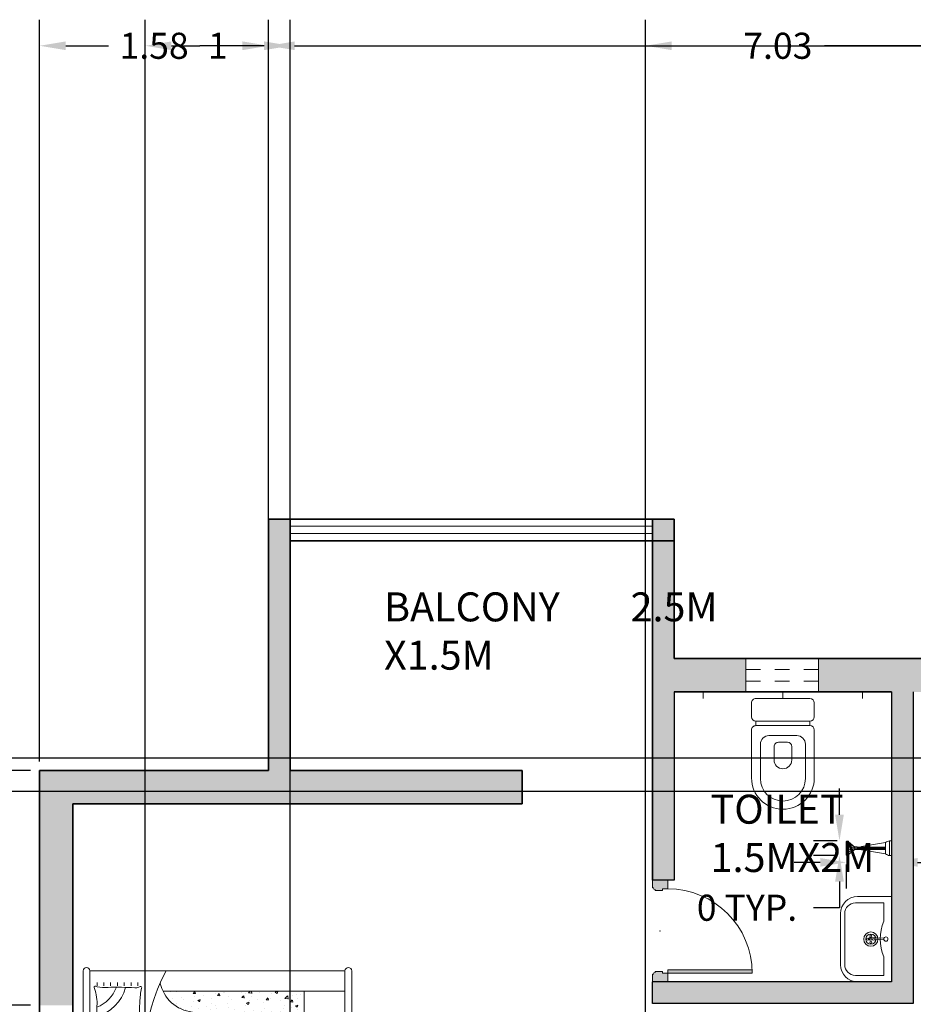
# Model space of a CAD drawing. Units: metres. Extents: x 2031 to 2061.8, y 1886.4 to 1909.8.
# Tile 6 of 10: x 2036.1 to 2042.3, y 1903 to 1909.8. Entities that reach past the tile are written whole.
import ezdxf

# ---------------------------------------------------------------- set-up
doc = ezdxf.new("R2010")
doc.units = ezdxf.units.M
doc.linetypes.add('DASHED', pattern=[0.75, 0.5, -0.25])
for name, color, linetype, lineweight in [('A-ANNO-DIMS', 2, 'Continuous', 18), ('A-AREA-IDEN', 7, 'Continuous', 18), ('A-FLOR-FIXT', 8, 'Continuous', 18), ('A-GLAZ-OVHD', 30, 'DASHED', 13), ('A-WALL-PATT', 252, 'Continuous', 13), ('doors & windows', 30, 'Continuous', 18), ('furniture', 24, 'Continuous', 13), ('grills', 5, 'Continuous', 13), ('inner walls', 4, 'Continuous', 25), ('windows', 30, 'Continuous', 18)]:
    doc.layers.add(name, color=color, linetype=linetype, lineweight=lineweight)
doc.layers.add('outer walls', color=1, linetype='Continuous', lineweight=35, plot=False)
doc.styles.get("Standard").update_dxf_attribs({"font": 'arial.ttf'})
doc.dimstyles.get("Standard").update_dxf_attribs({"dimtxt": 0.18, "dimasz": 0.18, "dimexe": 0.18, "dimexo": 0.0625, "dimgap": 0.09, "dimtad": 0, "dimtih": 1, "dimtoh": 1, "dimdec": 4, "dimzin": 0, "dimdsep": 46, "dimtxsty": 'Standard', "dimcen": 0.09, "dimadec": 0, "dimazin": 0, "dimtfac": 1, "dimtdec": 4, "dimtofl": 0, "dimtmove": 0, "dimatfit": 3, "dimfxl": 1, "dimtolj": 1, "dimtzin": 0, "dimarcsym": 0})

# ---------------------------------------------------------------- blocks, each defined once
blk = doc.blocks.new('D2')
at = {"layer": 'doors & windows'}
h = blk.add_hatch(dxfattribs=at)
h.set_pattern_fill('DOTS', color=256, scale=2, angle=180, style=0)
h.set_pattern_definition([(180, (0, -3.999999999998181), (-0.0625, -0.125), [0, -0.125])])
h.paths.add_polyline_path([(2.5, 1.819e-12), (3.5, 1.819e-12), (3.500000000001818, 24.97999199359535, 0.0100030022021123), (2.500000000001818, 25.00000000000182)])
h = blk.add_hatch(dxfattribs=at)
h.set_pattern_fill('DOTS', color=256, scale=2, angle=180, style=0)
h.set_pattern_definition([(180, (0, 0), (-0.0625, -0.125), [0, -0.125])])
edge = h.paths.add_edge_path()
edge.add_line((27.50000000000182, 1.819e-12), (27.50000000000182, -1.499999999998181))
edge.add_line((27.50000000000182, -1.499999999998181), (27.00000000000157, -1.499999999998181))
edge.add_line((27.00000000000157, -1.499999999998181), (27.00000000000039, -3.749999999998181))
edge.add_line((27.00000000000039, -3.749999999998181), (27.25, -3.749999999998181))
edge.add_arc((27.75893604593965, -3.741063954058532), 0.5090144907305875, 181.0059124648427, 268.9940875351573)
edge.add_line((27.75, -4.249999999998181), (27.75, -4.499999999998181))
edge.add_line((27.75, -4.499999999998181), (30.00000000000182, -4.499999999998181))
edge.add_line((30.00000000000182, -4.499999999998181), (30.00000000000182, 0))
edge.add_line((30.00000000000182, 0), (27.50000000000182, 1.819e-12))
edge = h.paths.add_edge_path()
edge.add_line((2.5, -1.499999999998181), (2.5, 1.819e-12))
edge.add_line((2.5, 1.819e-12), (1.819e-12, 0))
edge.add_line((1.819e-12, 0), (0, -4.499999999998181))
edge.add_line((0, -4.499999999998181), (2.250000000001548, -4.499999999998181))
edge.add_line((2.250000000001548, -4.499999999998181), (2.250000000001548, -4.249999999998181))
edge.add_arc((2.2410639540619, -3.741063954058532), 0.5090144907305875, 271.0059124648427, 358.9940875351573)
edge.add_line((2.750000000001548, -3.749999999998181), (3, -3.749999999998181))
edge.add_line((3, -3.749999999998181), (3, -1.499999999998181))
edge.add_line((3, -1.499999999998181), (2.5, -1.499999999998181))
for p, q in [((1.819e-12, 0), (0, -4.499999999998181)), ((30.00000000000182, 0), (30.00000000000182, -4.499999999998181))]:
    blk.add_line(p, q)
blk.add_lwpolyline([(3.5, 1.819e-12), (3.500000000001818, 25.00000000000182), (2.500000000001818, 25.00000000000182), (2.5, 1.819e-12)], close=True, dxfattribs=at)
for points in [[(3, -3.749999999998181), (3, -1.499999999998181), (2.5, -1.499999999998181), (2.5, 1.819e-12), (1.819e-12, 0)], [(27.00000000000039, -3.749999999998181), (27.00000000000182, -1.499999999998181), (27.50000000000182, -1.499999999998181), (27.50000000000182, 1.819e-12), (30, 0)], [(0, -4.499999999998181), (2.250000000001548, -4.499999999998181)], [(30, -4.499999999998181), (27.75, -4.499999999998181)]]:
    blk.add_lwpolyline(points, dxfattribs=at)
for points in [[(2.250000000001548, -4.499999999998181), (2.250000000001548, -4.249999999998181, 0.4039662087126686), (2.750000000001548, -3.749999999998181), (3.000000000001548, -3.749999999998181)], [(27.75, -4.499999999998181), (27.75, -4.249999999998181, -0.4039662087126686), (27.25, -3.749999999998181), (27, -3.749999999998181)]]:
    blk.add_lwpolyline(points, format="xyb", dxfattribs=at)
at = {"layer": 'doors & windows', "ltscale": 6}
blk.add_arc((2.5, 1.819e-12), 25, 0, 90, dxfattribs=at)
at = {"layer": 'doors & windows'}
blk.add_point((15, -2.24999999999909), dxfattribs=at)
blk = doc.blocks.new('wash basin 1')
for p, q in [((2.4e-15, 10), (-8, 10)), ((2.4e-15, 10), (-2.4e-15, -10)), ((-8.5, 8.5), (-1.851811242548834, 8.500000000000004)), ((-1.851811242548834, 8.500000000000004), (-1.851811242548897, 4.188089367671713)), ((-12, 6), (-12, -6.000000000000001)), ((-11, 6), (-11, -6.000000000000001)), ((-1.851811242548729, -8.5), (-1.851811242548728, -4.188089367671126)), ((-8.500000000000002, -8.500000000000002), (-1.851811242548729, -8.5)), ((-2.4e-15, -10), (-8.000000000000002, -10))]:
    blk.add_line(p, q)
blk.add_lwpolyline([(-1.829996854681013, 0.1082389988048371), (-5.253671435714977, 0.2462926470149123), (-5.229221238307189, -0.3815455523157976), (-1.804400006573047, -0.1898693366394459)])
for centre, radius in [((-4.868871099337752, 1.8e-15), 1.677439688297454), ((-4.868871099337752, 1.8e-15), 1.177439688297454), ((-5.631604960595723, 1.8e-15), 0.25), ((-4.873580145140294, 0.7523876361110525), 0.25), ((-4.868871099337752, 1.8e-15), 0.25), ((-4.194973017078154, 1.8e-15), 0.25), ((-1.341853106244229, 7.967e-13), 0.5), ((-4.868871099337752, -0.7188855560125376), 0.25)]:
    blk.add_circle(centre, radius)
for centre, radius, start, end in [((-8, 6), 4, 90, 180), ((-8.5, 6), 2.5, 90, 180), ((8.8933346853213, 5.103e-13), 11.53248687676786, 158.7058692194464, 201.2941307805559), ((-8.000000000000002, -6.000000000000001), 4, 180, 270), ((-8.500000000000002, -6.000000000000001), 2.5, 180, 270)]:
    blk.add_arc(centre, radius, start, end)
blk = doc.blocks.new('commode')
for p, q in [((-7.091161676878982, 19.40883832311374), (-7.091161676878982, 8.608954493363852)), ((-5.091161676878982, 11.8123055313481), (-5.091161676878982, 19.56719258349039)), ((5.091161676893534, 11.8123055313481), (5.091161676893534, 19.56719258349039)), ((7.091161676893534, 19.40883832311374), (7.091161676893534, 8.608954493363852)), ((-1.999999999985448, 12.37086546904174), (-1.999999999985448, 15.37086546904174)), ((2.000000000014551, 12.37086546904174), (2.000000000014551, 15.37086546904174)), ((-0.999999999985448, 11.37086546904174), (1.000000000014551, 11.37086546904174)), ((-3.149721614536247, 9.870865469041746), (3.149721614565351, 9.870865469041746)), ((-6.091161676878982, 7.608954493363853), (6.091161676893534, 7.608954493363853)), ((-6.091161676878982, 6.608954493363853), (-6.091161676878982, 7.608954493363851)), ((6.091161676893534, 7.608954493363854), (6.091161676893534, 6.608954493363853)), ((-7.091161676878982, 2.5), (-7.091161676878982, 5.608954493363853)), ((-6.091161676878982, 6.608954493363853), (6.091161676893534, 6.608954493363853)), ((7.091161676893534, 2.5), (7.091161676893534, 5.608954493363853)), ((-18, 1.5), (-18, 0)), ((-6.091161676878982, 1.5), (6.091161676893534, 1.5)), ((0, 1.5), (0, 0)), ((18, 1.5), (18, 0))]:
    blk.add_line(p, q)
for centre, radius, start, end in [((7.276e-12, 19.40883832311374), 7.091161676886258, 0, 180), ((7.276e-12, 19.56719258349039), 5.091161676886258, 0, 180), ((7.276e-12, 15.37086546904174), 2, 0, 180), ((-3.149721614536247, 11.8123055313481), 1.941440062334415, 180, 270), ((-0.999999999985448, 12.37086546904174), 1, 180, 270), ((1.000000000014551, 12.37086546904174), 1, 270, 0), ((3.149721614565351, 11.8123055313481), 1.941440062334415, 270, 0), ((-6.091161676878982, 8.608954493363852), 1, 180, 270), ((6.091161676893534, 8.608954493363852), 1, 270, 0), ((-6.091161676878982, 5.608954493363853), 1, 90, 180), ((6.091161676893534, 5.608954493363853), 1, 0, 90), ((-6.091161676878982, 2.5), 1, 180, 270), ((6.091161676893534, 2.5), 1, 270, 0)]:
    blk.add_arc(centre, radius, start, end)
blk = doc.blocks.new('tap & shower')
for p, q in [((1.708172111072059, 0), (-1.708172111072059, 0)), ((-1.708172111072059, 0), (-1.708166955903891, -0.5000109134438162)), ((1.708172111072059, 0), (1.708172111072059, -0.5)), ((1.708172111072059, -0.5), (-1.708172111072059, -0.5)), ((1.30544807404803, -1.402724037024029), (-1.30544807404803, -1.402724037024029)), ((-1.305442878530783, -1.402734990816952), (-0.3920875420875518, -6.99797979797978)), ((-0.3171055409637802, -0.5), (0.3171055409637802, -0.5)), ((-0.269360269360277, -7.941077441077368), (-0.269360269360277, -1.402724037024029)), ((-0.2154882154882216, -7.941077441077368), (-0.2154882154882216, -1.402724037024029)), ((-0.1616161616161662, -7.941077441077368), (-0.1616161616161662, -1.402724037024029)), ((0, -8.47979797979798), (0, -1.402724037024029)), ((0.1616161616161662, -7.941077441077425), (0.1616161616161662, -1.402724037024029)), ((0.2154882154882216, -7.941077441077425), (0.2154882154882216, -1.402724037024029)), ((0.269360269360277, -7.941077441077425), (0.269360269360277, -1.402724037024029)), ((0.3920875420875234, -6.99797979797978), (1.30544807404803, -1.402724037024029)), ((-1.481481481481495, -9.961279461279444), (-0.269360269360277, -8.47979797979798)), ((-0.2141589775469583, -8.47979797979798), (-0.9427609427609411, -9.961279461279444)), ((-0.0948641971181132, -8.47979797979798), (-0.4040404040404156, -9.961279461279444)), ((-0.3232323232323324, -7.941077441077368), (0.3232323232323324, -7.941077441077482)), ((-0.3232323232323324, -8.47979797979798), (-0.3232323232323324, -7.941077441077368)), ((-0.3232323232323324, -8.47979797979798), (0.3232323232323324, -8.47979797979798)), ((0.0948641971181132, -8.47979797979798), (0.4040404040404156, -9.961279461279444)), ((0.2141589775469583, -8.47979797979798), (0.9427609427609411, -9.961279461279444)), ((1.481481481481466, -9.961279461279444), (0.269360269360277, -8.47979797979798)), ((0.3232323232323324, -8.47979797979798), (0.3232323232323324, -7.941077441077482)), ((-1.616161616161605, -10.36531986531986), (-1.616161616161605, -10.09595959595958)), ((-1.481481481481495, -9.961279461279444), (1.481481481481466, -9.961279461279444)), ((-1.481481481481495, -10.5), (-1.481481481481495, -9.961279461279444)), ((-1.481481481481495, -10.5), (1.481481481481466, -10.5)), ((-1.427609427609439, -10.5), (-1.427609427609439, -9.961279461279444)), ((-1.373737373737384, -10.5), (-1.373737373737384, -9.961279461279444)), ((-1.319865319865328, -10.5), (-1.319865319865328, -9.961279461279444)), ((-1.265993265993273, -10.5), (-1.265993265993273, -9.961279461279444)), ((-1.212121212121218, -10.5), (-1.212121212121218, -9.961279461279444)), ((-1.158249158249162, -10.5), (-1.158249158249162, -9.961279461279444)), ((-1.104377104377107, -10.5), (-1.104377104377107, -9.961279461279444)), ((-1.050505050505051, -10.5), (-1.050505050505051, -9.961279461279444)), ((-0.9966329966329965, -10.5), (-0.9966329966329965, -9.961279461279444)), ((-0.9427609427609411, -10.5), (-0.9427609427609411, -9.961279461279444)), ((-0.8888888888888857, -10.5), (-0.8888888888888857, -9.961279461279444)), ((-0.8350168350168303, -10.5), (-0.8350168350168303, -9.961279461279444)), ((-0.781144781144775, -10.5), (-0.781144781144775, -9.961279461279444)), ((-0.7272727272727196, -10.5), (-0.7272727272727196, -9.961279461279444)), ((-0.6734006734006642, -10.5), (-0.6734006734006642, -9.961279461279444)), ((-0.6195286195286088, -10.5), (-0.6195286195286088, -9.961279461279444)), ((-0.5656565656565534, -10.5), (-0.5656565656565534, -9.961279461279444)), ((-0.5117845117845264, -10.5), (-0.5117845117845264, -9.961279461279444)), ((-0.457912457912471, -10.5), (-0.457912457912471, -9.961279461279444)), ((-0.4040404040404156, -10.5), (-0.4040404040404156, -9.961279461279444)), ((-0.3501683501683601, -10.5), (-0.3501683501683601, -9.961279461279444)), ((-0.2962962962963047, -10.5), (-0.2962962962963047, -9.961279461279444)), ((-0.2424242424242493, -10.5), (-0.2424242424242493, -9.961279461279444)), ((-0.1885521885521939, -10.5), (-0.1885521885521939, -9.961279461279444)), ((-0.1346801346801385, -10.5), (-0.1346801346801385, -9.961279461279444)), ((-0.0808080808080831, -10.5), (-0.0808080808080831, -9.961279461279444)), ((-0.0269360269360277, -10.5), (-0.0269360269360277, -9.961279461279444)), ((0.0269360269360277, -10.5), (0.0269360269360277, -9.961279461279444)), ((0.0808080808080831, -10.5), (0.0808080808080831, -9.961279461279444)), ((0.1346801346801385, -10.5), (0.1346801346801385, -9.961279461279444)), ((0.1885521885521939, -10.5), (0.1885521885521939, -9.961279461279444)), ((0.2424242424242493, -10.5), (0.2424242424242493, -9.961279461279444)), ((0.2962962962963047, -10.5), (0.2962962962963047, -9.961279461279444)), ((0.3501683501683601, -10.5), (0.3501683501683601, -9.961279461279444)), ((0.4040404040404156, -10.5), (0.4040404040404156, -9.961279461279444)), ((0.4579124579124425, -10.5), (0.4579124579124425, -9.961279461279444)), ((0.5117845117844979, -10.5), (0.5117845117844979, -9.961279461279444)), ((0.5656565656565534, -10.5), (0.5656565656565534, -9.961279461279444)), ((0.6195286195286088, -10.5), (0.6195286195286088, -9.961279461279444)), ((0.6734006734006642, -10.5), (0.6734006734006642, -9.961279461279444)), ((0.7272727272727196, -10.5), (0.7272727272727196, -9.961279461279444)), ((0.781144781144775, -10.5), (0.781144781144775, -9.961279461279444)), ((0.8350168350168303, -10.5), (0.8350168350168303, -9.961279461279444)), ((0.8888888888888857, -10.5), (0.8888888888888857, -9.961279461279444)), ((0.9427609427609411, -10.5), (0.9427609427609411, -9.961279461279444)), ((0.9966329966329965, -10.5), (0.9966329966329965, -9.961279461279444)), ((1.050505050505051, -10.5), (1.050505050505051, -9.961279461279444)), ((1.104377104377107, -10.5), (1.104377104377107, -9.961279461279444)), ((1.158249158249162, -10.5), (1.158249158249162, -9.961279461279444)), ((1.212121212121218, -10.5), (1.212121212121218, -9.961279461279444)), ((1.265993265993273, -10.5), (1.265993265993273, -9.961279461279444)), ((1.319865319865328, -10.5), (1.319865319865328, -9.961279461279444)), ((1.373737373737384, -10.5), (1.373737373737384, -9.961279461279444)), ((1.427609427609439, -10.5), (1.427609427609439, -9.961279461279444)), ((1.481481481481466, -10.5), (1.481481481481466, -9.961279461279444)), ((1.616161616161605, -10.36531986531986), (1.616161616161605, -10.09595959595958))]:
    blk.add_line(p, q)
for centre, radius, start, end in [((-0.0174713202327155, -0.2869501082291208), 1.704067674476668, 187.1825297220346, 220.9027681176297), ((0.0174793747132753, -0.2869501082291208), 1.704067674476639, 319.0972318823703, 352.8174702779653), ((0, -6.985663239740574), 0.3922809430333202, 181.7992278553774, 358.2007721446227), ((-1.481481481481495, -10.09595959595958), 0.1346801346801346, 90, 180), ((-1.481481481481495, -10.36531986531986), 0.1346801346801346, 180, 270), ((1.481481481481466, -10.09595959595958), 0.1346801346801346, 0, 90), ((1.481481481481466, -10.36531986531986), 0.1346801346801346, 270, 0)]:
    blk.add_arc(centre, radius, start, end)
blk = doc.blocks.new('bed')
at = {"layer": 'furniture'}
h = blk.add_hatch(dxfattribs=at)
h.set_pattern_fill('AR-CONC', color=256, angle=-90.00000000000003, style=0)
h.set_pattern_definition([(320, (0, 2.380000000001032), (-0.6275213498259539, -7.172601826007534), [0.75, -8.25]), (265, (0, 2.380000000001032), (7.521921337000119, 1.387513336129997), [0.6, -6.599999999999999]), (10.45139999999999, (-0.0522933999999964, 1.782283200001032), (6.894395420609534, -5.785093817140218), [0.6374019000000001, -7.011421119999999]), (316.1842, (2, 2.380000000001032), (-1.655190143290184, -10.67241048625644), [1.125, -12.375]), (6.635599999999979, (1.862066929999997, 1.490632550001038), (9.741178709004412, -9.346627055487035), [0.956102879999999, -10.51712999999998]), (261.1842, (2, 2.380000000001032), (9.741186009253243, -9.346619451336275), [0.8999999999999989, -9.899999999999984]), (291, (1.5, 1.380000000001032), (-4.02618890665339, -5.969070521184614), [0.75, -8.25]), (236, (1.5, 1.380000000001032), (7.251500450468529, -2.433153319215819), [0.6, -6.599999999999999]), (341.4514, (1.164483939999996, 0.8825776700010266), (3.22530496709952, -8.402226285814901), [0.6374019000000001, -7.011421119999999]), (307.4999999999999, (0, 2.380000000001032), (3.328938538313114, -0.121598553172908), [0, -6.519999999999999, 0, -6.7, 0, -6.625]), (277.5, (0, 2.380000000001032), (3.944117118823601, -2.630695374421487), [0, -3.819999999999999, 0, -6.37, 0, -2.524999999999999]), (237.5, (0, 4.610000000001036), (-0.2255487173438, -5.33822436172409), [0, -2.5, 0, -7.799999999999999, 0, -10.35]), (227.5, (0, 5.610000000001036), (1.001049823323174, -5.831861693423862), [0, -3.25, 0, -5.179999999999999, 0, -7.349999999999999])])
h.paths.add_polyline_path([(30.01221964123038, -67.99999999999999), (30.01221964123036, -26.4972098666525, 0.2630430180581192), (23.90476957024844, -35.1500155485824, 0.2934236934375176), (-9.177957282599145, -26.46678060096597, -0.1566832162072435), (-23.39221964123496, -28.71851562074189), (-23.39221964123494, -67.99999999999999)])
for p, q in [((0, -3), (0, 0)), ((36.01221964123033, -3), (-36.01221964123033, -3)), ((-36.01221964123033, -5.000000000000028), (-36.01221964123027, -80)), ((36.01221964123033, -5.000000000000042), (-36.01221964123033, -5.000000000000028)), ((0, -8.000000000000043), (0, -5.000000000000042)), ((36.01221964123039, -79.99999999999999), (36.01221964123033, -5.000000000000042)), ((-31.23716250644156, -7.067621994530554), (-32.23716250644157, -7.067621994530554)), ((-3.810600647213163, -7.067621994530554), (-2.810600647213163, -7.067621994530554)), ((3.894900133777696, -7.067621994530526), (2.894900133777696, -7.067621994530526)), ((31.62837541028949, -7.067621994530526), (32.62837541028949, -7.067621994530526)), ((-31.23716250644156, -9.067621994530555), (-32.23716250644157, -9.067621994530555)), ((-31.23716250644156, -11.06762199453055), (-32.23716250644157, -11.06762199453055)), ((-3.810600647213163, -9.067621994530555), (-2.810600647213163, -9.067621994530555)), ((-3.810600647213163, -11.06762199453055), (-2.810600647213163, -11.06762199453055)), ((3.894900133777696, -9.067621994530526), (2.894900133777696, -9.067621994530526)), ((3.894900133777696, -11.06762199453052), (2.894900133777696, -11.06762199453052)), ((31.62837541028949, -9.067621994530526), (32.62837541028949, -9.067621994530526)), ((31.62837541028949, -11.06762199453052), (32.62837541028949, -11.06762199453052)), ((-31.23716250644156, -13.06762199453055), (-32.23716250644157, -13.06762199453055)), ((-3.810600647213163, -13.06762199453055), (-2.810600647213163, -13.06762199453055)), ((3.894900133777696, -13.06762199453052), (2.894900133777696, -13.06762199453052)), ((31.62837541028949, -13.06762199453052), (32.62837541028949, -13.06762199453052)), ((-31.23716250644156, -15.06762199453055), (-32.23716250644157, -15.06762199453055)), ((-31.23716250644156, -17.06762199453055), (-32.23716250644157, -17.06762199453055)), ((-3.810600647213163, -15.06762199453055), (-2.810600647213163, -15.06762199453055)), ((-3.810600647213163, -17.06762199453055), (-2.810600647213163, -17.06762199453055)), ((3.894900133777696, -15.06762199453052), (2.894900133777696, -15.06762199453052)), ((3.894900133777696, -17.06762199453052), (2.894900133777696, -17.06762199453052)), ((31.62837541028949, -15.06762199453052), (32.62837541028949, -15.06762199453052)), ((31.62837541028949, -17.06762199453052), (32.62837541028949, -17.06762199453052)), ((-31.23716250644156, -19.06762199453055), (-32.23716250644157, -19.06762199453055)), ((-3.810600647213163, -19.06762199453055), (-2.810600647213163, -19.06762199453055)), ((3.894900133777696, -19.06762199453052), (2.894900133777696, -19.06762199453052)), ((31.62837541028949, -19.06762199453052), (32.62837541028949, -19.06762199453052)), ((-36.01221964123027, -80), (36.01221964123039, -79.99999999999997)), ((-36.01221964123027, -82), (36.01221964123039, -82))]:
    blk.add_line(p, q, dxfattribs=at)
at = {"layer": 'furniture', "ltscale": 5}
blk.add_line((-30.0122196412303, -26.65900214866815), (-30.01221964123028, -80), dxfattribs=at)
at = {"layer": 'furniture', "ltscale": 0.3}
for p, q in [((-23.39221964123493, -80.00000000000003), (-23.39221964123496, -28.71851562074188)), ((-30.01221964123028, -67.99999999999999), (30.01221964123039, -67.99999999999999))]:
    blk.add_line(p, q, dxfattribs=at)
at = {"layer": 'furniture', "ltscale": 7}
blk.add_line((30.01221964123039, -79.99999999999999), (30.01221964123036, -26.4972098666525), dxfattribs=at)
at = {"layer": 'furniture'}
for centre, radius, start, end in [((-35.95310404783035, -4.000000000000014), 1.001745802777857, 93.38313670775338, 266.6168632922466), ((35.95310404783047, -4.000000000000014), 1.001745802777857, 273.3831367077534, 86.61686329224663), ((-31.09685452420217, -6.56812628935117), 0.3815901177143176, 35.89755946985184, 208.6271807330242), ((-44.4434251214767, -13.85312857714783), 14.82374463825802, 27.16285943351717, 28.62718073212637), ((-46.75951437957865, -9.65138206848897), 15.71579241958107, 357.4803608088326, 9.395608387614068), ((-34.45294545533051, -3.506108501804959), 9.853247350176973, 289.8695209624031, 338.9842964810487), ((-34.45294545533051, -3.506108501804959), 12.47479548168961, 286.0319050224358, 344.1205283884622), ((-26.34909713879518, 6.677823774407073), 13.75788850886336, 251.1782289026713, 273.3982224065857), ((-18.01528168092849, -163.5963416214672), 156.7209082093599, 87.00321809951629, 92.74968346925495), ((-8.031939823939297, 2.030581047412752), 9.294330538692307, 258.8960367609226, 294.7184225587751), ((0.254091396095987, -8.800915214962217), 4.494229367051207, 159.014640107615, 186.2730421081171), ((-4.029449448298862, -6.668977911985379), 0.2818061021667602, 335.7259061638442, 114.3030308467571), ((3.223958981487498, -9.94006998173215), 7.675076275868892, 155.7259061638442, 159.0146401085631), ((4.113748934860268, -6.668977911985379), 0.2818061021635516, 65.69696915417202, 204.2740938370052), ((-3.139659494904833, -9.940069981732137), 7.675076275868892, 20.98535989143595, 24.27409383615427), ((-0.1697919095242355, -8.800915214962217), 4.494229367051207, 353.7269578918828, 20.98535989238499), ((8.116239310533615, 2.030581047735168), 9.294330539002221, 245.2815774418415, 281.1039632384965), ((18.09958116748922, -163.5963416214399), 156.7209082093326, 87.2503165307418, 92.99678190048373), ((34.53724494190226, -3.506108501789682), 12.47479548168961, 195.8794716115377, 253.9680949775642), ((34.53724494190226, -3.506108501789682), 9.853247350176973, 201.0157035189505, 250.1304790375968), ((26.43339662535652, 6.677823774423444), 13.75788850886336, 266.6017775934111, 288.8217710973251), ((31.18115401076358, -6.568126289351184), 0.3815901177179044, 331.3728192669758, 144.1024405301472), ((46.84381386614001, -9.651382068520647), 15.71579241958353, 170.6043916115409, 182.5196391911672), ((44.52772460803806, -13.85312857714784), 14.82374463825802, 151.3728192678729, 152.8371405664821), ((-28.61556435462791, 31.03444768063454), 42.31456350822244, 266.4835611990511, 266.6487421238194), ((54.88285648445511, -13.16191061182081), 85.98801403775587, 178.1208768196816, 183.3613129440673), ((-32.81622258778788, -12.43616332427339), 28.77528664700029, 354.3784002715227, 6.27304210895588), ((32.90052207435963, -12.43616332427341), 28.77528664700055, 173.7269578910441, 185.6215997284773), ((-54.79855699787332, -13.1619106118885), 85.98801403775471, 356.6386870559327, 1.87912318031836), ((28.69986384117891, 31.03444768073385), 42.31456350831875, 273.3512578762066, 273.5164388009489), ((12.27920019974715, -16.10835590841725), 16.48064095036883, 177.0317121189266, 192.8677860199701), ((-12.19490071317551, -16.10835590841725), 16.48064095036894, 347.1322139800299, 2.968287881073314), ((-31.05019458355673, -19.91479358257859), 0.2912925215689113, 147.6219291273817, 311.93432899363), ((-33.19532486499685, -18.55460390606353), 2.248727139855352, 327.6219291288709, 339.224552802207), ((-34.12771521855714, -18.41167218428833), 3.177308659740759, 342.7808628527732, 3.755021134780372), ((-24.39731400277299, -58.0065508966982), 38.42172354635978, 93.51643880178425, 99.67664784205135), ((-24.51665474671893, -56.06449133928439), 36.47600066328987, 86.48356119821578, 93.51643880178425), ((-18.48842024981553, 70.49496359167773), 90.23180174042126, 267.5920770069633, 273.6328801943956), ((-10.30534078399284, -44.95285539311296), 25.51674577343078, 75.95197577712642, 95.54518109318596), ((-3.947726608991956, -19.99033763805275), 0.2654728058058112, 231.9004795059564, 52.89022406852256), ((4.032026095563765, -19.99033763805275), 0.2654728058058112, 127.1097759314774, 308.0995204940429), ((7.570216687580227, -34.67789736270967), 14.86666553287629, 87.39755039330738, 103.1191401867811), ((11.43897390287765, -34.80624327566366), 15.31635237680183, 84.69404282866213, 102.035481886755), ((18.57271973638731, 70.4949635916777), 90.23180174042125, 266.3671198056044, 272.4079229930367), ((24.6009542333012, -56.0644913392844), 36.47600066328987, 86.48356119821578, 93.51643880178425), ((24.48161348934542, -58.00655089669821), 38.42172354635978, 80.32335215794863, 86.48356119821578), ((31.13449407013883, -19.91479358255678), 0.2912925215689113, 228.06567100637, 32.37807087261824), ((34.21201470513921, -18.41167218428845), 3.177308659740705, 176.2449788652196, 197.2191371472267), ((33.27962435157895, -18.55460390604825), 2.248727139855352, 200.775447197793, 212.378070871129), ((-19.78970084288576, -5.469494448941333), 23.52647715105876, 226.4060518471351, 297.4441169484015), ((12.50744191168894, -69.71437404891591), 48.3828132966499, 60.93454900685955, 116.3226601669859), ((0.602167516954296, -56.56840710701565), 31.65057281321388, 42.58740832788977, 108.5033645785765), ((34.6132349005153, -36.22659364526982), 10.76244628919441, 101.1719081394, 174.2590453022261), ((-35.95310404783035, -81), 1.001745802777857, 93.38313670775338, 266.6168632922466), ((35.95310404783044, -81), 1.001745802777857, 273.3831367077534, 86.61686329224663)]:
    blk.add_arc(centre, radius, start, end, dxfattribs=at)
blk = doc.blocks.new('BALCONY-GUARD-2500')
for p, q in [((4.547e-13, 0.0500000000010914), (2.5, 0.0500000000006367)), ((4.547e-13, 6.821e-13), (2.5, 4.547e-13))]:
    blk.add_line(p, q)
blk = doc.blocks.new('*D32')
at = {"layer": 'A-ANNO-DIMS', "color": 0, "lineweight": -2, "transparency": 16777216}
for p, q in [((2041.621106728857, 1904.024726820454), (2041.441106728857, 1904.024726820454)), ((2041.801106728857, 1904.009143718862), (2041.801106728857, 1903.844726820454)), ((2042.113886051581, 1904.009143718862), (2042.113886051581, 1903.844726820454)), ((2042.293886051581, 1904.024726820454), (2042.473886051581, 1904.024726820454))]:
    blk.add_line(p, q, dxfattribs=at)
at = {"layer": 'A-ANNO-DIMS', "color": 0, "transparency": 16777216}
for points in [[(2041.621106728857, 1904.054726820454), (2041.621106728857, 1903.994726820454), (2041.801106728857, 1904.024726820454)], [(2042.293886051581, 1904.054726820454), (2042.293886051581, 1903.994726820454), (2042.113886051581, 1904.024726820454)]]:
    blk.add_solid(points, dxfattribs=at)
at = {"layer": 'Defpoints', "color": 0, "transparency": 16777216}
for p in [(2041.801106728857, 1904.071643718862), (2042.113886051581, 1904.071643718862), (2042.113886051581, 1904.024726820454)]:
    blk.add_point(p, dxfattribs=at)
at = {"layer": 'A-ANNO-DIMS', "color": 0, "transparency": 16777216, "insert": (2043.532337620476, 1904.024726820454), "char_height": 0.18, "attachment_point": 5}
blk.add_mtext('\\A1;SHOWER 0 TYP.', dxfattribs=at)
blk = doc.blocks.new('*D33')
at = {"layer": 'A-ANNO-DIMS', "color": 0, "lineweight": -2, "transparency": 16777216}
for p, q in [((2041.75418983045, 1904.353411598752), (2041.75418983045, 1904.533411598752)), ((2041.738606728858, 1904.173411598752), (2041.574189830451, 1904.173411598752)), ((2041.738606728858, 1904.071643718863), (2041.574189830451, 1904.071643718863)), ((2041.75418983045, 1903.891643718863), (2041.75418983045, 1903.711643718863)), ((2041.75418983045, 1903.711643718863), (2041.574189830451, 1903.711643718863))]:
    blk.add_line(p, q, dxfattribs=at)
at = {"layer": 'A-ANNO-DIMS', "color": 0, "transparency": 16777216}
for points in [[(2041.724189830451, 1904.353411598752), (2041.784189830451, 1904.353411598752), (2041.75418983045, 1904.173411598752)], [(2041.724189830451, 1903.891643718863), (2041.784189830451, 1903.891643718863), (2041.75418983045, 1904.071643718863)]]:
    blk.add_solid(points, dxfattribs=at)
at = {"layer": 'Defpoints', "color": 0, "transparency": 16777216}
for p in [(2041.801106728858, 1904.173411598752), (2041.75418983045, 1904.071643718863), (2041.801106728858, 1904.071643718863)]:
    blk.add_point(p, dxfattribs=at)
at = {"layer": 'A-ANNO-DIMS', "color": 0, "transparency": 16777216, "insert": (2041.116024755417, 1903.711643718862), "char_height": 0.18, "attachment_point": 5}
blk.add_mtext('\\A1;0 TYP.', dxfattribs=at)
blk = doc.blocks.new('*D46')
at = {"layer": 'A-ANNO-DIMS', "color": 0, "lineweight": -2, "transparency": 16777216}
for p, q in [((2036.233886, 1904.721924), (2036.233886, 1909.84065)), ((2037.813886, 1904.721924), (2037.813886, 1909.84065)), ((2036.413886, 1909.66065), (2036.708394867667, 1909.66065)), ((2037.633886, 1909.66065), (2037.339377132333, 1909.66065))]:
    blk.add_line(p, q, dxfattribs=at)
at = {"layer": 'A-ANNO-DIMS', "color": 0, "transparency": 16777216}
for points in [[(2036.413886, 1909.69065), (2036.413886, 1909.63065), (2036.233886, 1909.66065)], [(2037.633886, 1909.69065), (2037.633886, 1909.63065), (2037.813886, 1909.66065)]]:
    blk.add_solid(points, dxfattribs=at)
at = {"layer": 'Defpoints', "color": 0, "transparency": 16777216}
for p in [(2037.813886, 1909.66065), (2036.233886, 1904.659424), (2037.813886, 1904.659424)]:
    blk.add_point(p, dxfattribs=at)
at = {"layer": 'A-ANNO-DIMS', "color": 0, "transparency": 16777216, "insert": (2037.023886, 1909.66065), "char_height": 0.18, "attachment_point": 5}
blk.add_mtext('\\A1;1.58', dxfattribs=at)
blk = doc.blocks.new('*D47')
at = {"layer": 'A-ANNO-DIMS', "color": 0, "lineweight": -2, "transparency": 16777216}
for p, q in [((2037.813886, 1906.456584), (2037.813886, 1909.84065)), ((2044.843886, 1907.143703), (2044.843886, 1909.84065)), ((2037.993886, 1909.66065), (2041.005843708049, 1909.66065)), ((2044.663886, 1909.66065), (2041.651928291951, 1909.66065))]:
    blk.add_line(p, q, dxfattribs=at)
at = {"layer": 'A-ANNO-DIMS', "color": 0, "transparency": 16777216}
for points in [[(2037.993886, 1909.69065), (2037.993886, 1909.63065), (2037.813886, 1909.66065)], [(2044.663886, 1909.69065), (2044.663886, 1909.63065), (2044.843886, 1909.66065)]]:
    blk.add_solid(points, dxfattribs=at)
at = {"layer": 'Defpoints', "color": 0, "transparency": 16777216}
for p in [(2044.843886, 1909.66065), (2044.843886, 1907.081203), (2037.813886, 1906.394084)]:
    blk.add_point(p, dxfattribs=at)
at = {"layer": 'A-ANNO-DIMS', "color": 0, "transparency": 16777216, "insert": (2041.328886, 1909.66065), "char_height": 0.18, "attachment_point": 5}
blk.add_mtext('\\A1;7.03', dxfattribs=at)
blk = doc.blocks.new('*D53')
at = {"layer": 'A-ANNO-DIMS', "color": 0, "lineweight": -2, "transparency": 16777216}
for p, q in [((2036.171386000001, 1904.659424000001), (2031.564780000002, 1904.659424000001)), ((2031.744780000002, 1904.479424000001), (2031.744780000002, 1904.031116637791)), ((2031.744780000002, 1903.219003000001), (2031.744780000002, 1903.667310362211)), ((2036.171386000001, 1903.039003000001), (2031.564780000002, 1903.039003000001))]:
    blk.add_line(p, q, dxfattribs=at)
at = {"layer": 'A-ANNO-DIMS', "color": 0, "transparency": 16777216}
for points in [[(2031.714780000002, 1904.479424000001), (2031.774780000002, 1904.479424000001), (2031.744780000002, 1904.659424000001)], [(2031.714780000002, 1903.219003000001), (2031.774780000002, 1903.219003000001), (2031.744780000002, 1903.039003000001)]]:
    blk.add_solid(points, dxfattribs=at)
at = {"layer": 'Defpoints', "color": 0, "transparency": 16777216}
for p in [(2031.744780000002, 1904.659424000001), (2036.233886000001, 1904.659424000001), (2036.233886000001, 1903.039003000001)]:
    blk.add_point(p, dxfattribs=at)
at = {"layer": 'A-ANNO-DIMS', "color": 0, "transparency": 16777216, "insert": (2031.744780000002, 1903.8492135), "char_height": 0.18, "attachment_point": 5}
blk.add_mtext('\\A1;1.62', dxfattribs=at)
blk = doc.blocks.new('*D58')
at = {"layer": 'A-ANNO-DIMS', "color": 0, "lineweight": -2, "transparency": 16777216}
for p, q in [((2040.415705, 1896.633713), (2040.415705, 1909.84065)), ((2052.040038, 1896.633713), (2052.040038, 1909.84065)), ((2040.595705, 1909.66065), (2045.773082959755, 1909.66065)), ((2051.860038, 1909.66065), (2046.682660040246, 1909.66065))]:
    blk.add_line(p, q, dxfattribs=at)
at = {"layer": 'A-ANNO-DIMS', "color": 0, "transparency": 16777216}
for points in [[(2040.595705, 1909.69065), (2040.595705, 1909.63065), (2040.415705, 1909.66065)], [(2051.860038, 1909.69065), (2051.860038, 1909.63065), (2052.040038, 1909.66065)]]:
    blk.add_solid(points, dxfattribs=at)
at = {"layer": 'Defpoints', "color": 0, "transparency": 16777216}
for p in [(2052.040038, 1909.66065), (2040.415705, 1896.571213), (2052.040038, 1896.571213)]:
    blk.add_point(p, dxfattribs=at)
at = {"layer": 'A-ANNO-DIMS', "color": 0, "transparency": 16777216, "insert": (2046.227871500001, 1909.66065), "char_height": 0.18, "attachment_point": 5}
blk.add_mtext('\\A1;11.624', dxfattribs=at)
blk = doc.blocks.new('*D59')
at = {"layer": 'A-ANNO-DIMS', "color": 0, "lineweight": -2, "transparency": 16777216}
for p, q in [((2036.963194, 1898.433713), (2036.963194, 1909.84065)), ((2037.963194, 1898.433713), (2037.963194, 1909.84065)), ((2037.143194, 1909.66065), (2037.340042567531, 1909.66065)), ((2037.783194, 1909.66065), (2037.586345432469, 1909.66065))]:
    blk.add_line(p, q, dxfattribs=at)
at = {"layer": 'A-ANNO-DIMS', "color": 0, "transparency": 16777216}
for points in [[(2037.143194, 1909.69065), (2037.143194, 1909.63065), (2036.963194, 1909.66065)], [(2037.783194, 1909.69065), (2037.783194, 1909.63065), (2037.963194, 1909.66065)]]:
    blk.add_solid(points, dxfattribs=at)
at = {"layer": 'Defpoints', "color": 0, "transparency": 16777216}
for p in [(2037.963194, 1909.66065), (2036.963194, 1898.371213), (2037.963194, 1898.371213)]:
    blk.add_point(p, dxfattribs=at)
at = {"layer": 'A-ANNO-DIMS', "color": 0, "transparency": 16777216, "insert": (2037.463194, 1909.66065), "char_height": 0.18, "attachment_point": 5}
blk.add_mtext('\\A1;1', dxfattribs=at)
blk = doc.blocks.new('*D60')
at = {"layer": 'A-ANNO-DIMS', "color": 0, "lineweight": -2, "transparency": 16777216}
for p, q in [((2031.744780000002, 1904.924084000001), (2031.744780000002, 1905.104084000001)), ((2056.161386000001, 1904.744084), (2031.564780000002, 1904.744084)), ((2055.931386000001, 1904.514084000001), (2031.564780000002, 1904.514084000001)), ((2031.744780000002, 1904.334084000001), (2031.744780000002, 1904.154084000001)), ((2031.744780000002, 1904.154084000001), (2031.564780000002, 1904.154084000001))]:
    blk.add_line(p, q, dxfattribs=at)
at = {"layer": 'A-ANNO-DIMS', "color": 0, "transparency": 16777216}
for points in [[(2031.714780000002, 1904.924084000001), (2031.774780000002, 1904.924084000001), (2031.744780000002, 1904.744084)], [(2031.714780000002, 1904.334084000001), (2031.774780000002, 1904.334084000001), (2031.744780000002, 1904.514084000001)]]:
    blk.add_solid(points, dxfattribs=at)
at = {"layer": 'Defpoints', "color": 0, "transparency": 16777216}
for p in [(2056.223886000001, 1904.744084), (2031.744780000002, 1904.514084000001), (2055.993886000001, 1904.514084000001)]:
    blk.add_point(p, dxfattribs=at)
at = {"layer": 'A-ANNO-DIMS', "color": 0, "transparency": 16777216, "insert": (2031.241001009552, 1904.154084), "char_height": 0.18, "attachment_point": 5}
blk.add_mtext('\\A1;0.23', dxfattribs=at)

msp = doc.modelspace()

# ---------------------------------------------------------------- hatches: boundary and pattern name
at = {"layer": 'A-WALL-PATT'}
h = msp.add_hatch(color=256, dxfattribs=at)
h.dxf.hatch_style = 1
h.paths.add_polyline_path([(2044.843886051581, 1905.431202972395), (2043.662726773602, 1905.431202972395), (2043.662726773602, 1905.201202972395), (2044.613886051581, 1905.201202972395), (2044.613886051581, 1903.201202972395), (2044.10203621828, 1903.201202972395), (2044.10203621828, 1903.051247813867), (2044.613886051581, 1903.051202972395), (2044.613784550147, 1901.892599367488), (2044.843481671829, 1901.892599367488)])
h.paths.add_polyline_path([(2044.843886051581, 1907.081202972395), (2044.693886051581, 1907.081202972395), (2044.693886051581, 1905.431202972395), (2044.843886051581, 1905.431202972395)])
h.paths.add_polyline_path([(2042.662726773602, 1905.431202972395), (2041.608725591668, 1905.431202972395), (2041.608725591668, 1905.201202972395), (2042.113886051581, 1905.201202972395), (2042.113886051581, 1903.201202972395), (2042.11388605158, 1903.200960518025), (2041.878665859902, 1903.200960518025, -0.0160568248018428), (2041.87111792116, 1903.201202972395), (2040.613886051581, 1903.201202972395), (2040.463886051581, 1903.201202972395), (2040.46388605158, 1903.051202972395), (2042.263886051581, 1903.051202972395), (2042.263886051581, 1905.201202972395), (2042.662726773602, 1905.201202972395)])
h.paths.add_polyline_path([(2040.804457664849, 1903.878793012381), (2041.776183449296, 1903.878793012381), (2041.776183449296, 1904.438513339803), (2040.804457664849, 1904.438513339803)], flags=25)
h.paths.add_polyline_path([(2042.05521314868, 1900.945611707966), (2043.754121743495, 1900.945611707966), (2043.754121743495, 1901.691905477861), (2042.05521314868, 1901.691905477861)], flags=9)
h.paths.add_polyline_path([(2038.540886554753, 1905.248744193212), (2040.159440442883, 1905.248744193212), (2040.159440442883, 1905.995037963107), (2038.540886554753, 1905.995037963107)], flags=9)
h.paths.add_polyline_path([(2038.693906317999, 1902.140700941841), (2040.392814912815, 1902.140700941841), (2040.392814912815, 1902.886994711737), (2038.693906317999, 1902.886994711737)], flags=9)
h.paths.add_polyline_path([(2042.359230799286, 1903.821641126969), (2043.685560949354, 1903.821641126969), (2043.685560949354, 1904.567934896864), (2042.359230799286, 1904.567934896864)], flags=9)
h = msp.add_hatch(color=256, dxfattribs=at)
h.dxf.hatch_style = 1
h.paths.add_polyline_path([(2037.96388605158, 1906.2440838694), (2037.96388605158, 1906.3940838694), (2037.81388605158, 1906.3940838694), (2037.81388605158, 1904.659423662096), (2036.233886051581, 1904.659423662097), (2036.233425041249, 1903.039002867159), (2036.463447491671, 1903.039002867159), (2036.463886051581, 1904.429423662097), (2039.563886051581, 1904.429423662097), (2039.563886051581, 1904.659423662097), (2037.96388605158, 1904.659423662097)])
h = msp.add_hatch(color=256, dxfattribs=at)
h.dxf.hatch_style = 1
h.paths.add_polyline_path([(2040.613886051581, 1906.394083869399), (2040.46388605158, 1906.394083869399), (2040.46388605158, 1906.2440838694), (2040.613886051581, 1906.2440838694)])
h = msp.add_hatch(color=256, dxfattribs=at)
h.dxf.hatch_style = 1
h.paths.add_polyline_path([(2040.613886051581, 1905.431202972395), (2040.613886051581, 1906.2440838694), (2040.46388605158, 1906.2440838694), (2040.46388605158, 1903.901202972395), (2040.613886051581, 1903.901202972395), (2040.613886051581, 1905.201202972395), (2041.108725591668, 1905.201202972395), (2041.108725591668, 1905.431202972395)])

# ---------------------------------------------------------------- linework, layer by layer
at = {"layer": 'A-GLAZ-OVHD', "ltscale": 0.2}
for p, q in [((2041.108725591668, 1905.356202972394), (2041.608725591668, 1905.356202972394)), ((2041.108725591668, 1905.276202972394), (2041.608725591668, 1905.276202972394))]:
    msp.add_line(p, q, dxfattribs=at)
at = {"layer": 'inner walls'}
for p, q in [((2040.613886051581, 1905.201202972395), (2040.613886051581, 1903.901202972395)), ((2042.113886051581, 1905.201202972395), (2042.113886051581, 1903.201202972395)), ((2042.263886051581, 1905.201202972395), (2042.263886051581, 1903.051202972395)), ((2040.613886051581, 1903.901202972395), (2040.46388605158, 1903.901202972395)), ((2040.613886051581, 1903.201202972395), (2040.46388605158, 1903.201202972395)), ((2040.46388605158, 1903.051202972395), (2040.463886051581, 1903.201202972395)), ((2042.113886051581, 1903.201202972395), (2040.613886051581, 1903.201202972395)), ((2042.263886051581, 1903.051202972395), (2040.46388605158, 1903.051202972395))]:
    msp.add_line(p, q, dxfattribs=at)
at = {"layer": 'outer walls'}
for p, q in [((2037.81388605158, 1906.3940838694), (2040.613886051581, 1906.394083869399)), ((2037.81388605158, 1906.3940838694), (2037.81388605158, 1904.659423662096)), ((2037.96388605158, 1906.2440838694), (2037.96388605158, 1906.3940838694)), ((2040.46388605158, 1906.244083869399), (2040.46388605158, 1906.394083869399)), ((2040.613886051581, 1906.394083869399), (2040.613886051581, 1905.431202972395)), ((2037.96388605158, 1906.2440838694), (2040.613886051581, 1906.2440838694)), ((2037.96388605158, 1906.2440838694), (2037.96388605158, 1904.659423662097)), ((2040.46388605158, 1906.244083869399), (2040.46388605158, 1903.901202972395)), ((2040.613886051581, 1905.431202972395), (2044.843886051581, 1905.431202972395)), ((2040.613886051581, 1905.201202972395), (2042.113886051581, 1905.201202972395)), ((2036.233886051581, 1904.659423662097), (2036.232783035539, 1900.782395301215)), ((2036.233886051581, 1904.659423662097), (2037.81388605158, 1904.659423662096)), ((2037.96388605158, 1904.659423662097), (2039.563886051581, 1904.659423662097)), ((2039.563886051581, 1904.429423662097), (2039.563886051581, 1904.659423662097)), ((2036.463886051581, 1904.429423662097), (2036.462783035539, 1900.932395301215)), ((2039.563886051581, 1904.429423662097), (2036.463886051581, 1904.429423662097))]:
    msp.add_line(p, q, dxfattribs=at)
at = {"layer": 'windows'}
for p, q in [((2041.108725591668, 1905.201202972395), (2041.108725591668, 1905.431202972394)), ((2041.608725591668, 1905.201202972395), (2041.608725591668, 1905.431202972395))]:
    msp.add_line(p, q, dxfattribs=at)

# ---------------------------------------------------------------- block references
at = {"layer": 'A-FLOR-FIXT'}
for name, p, xscale, yscale, zscale, rotation in [('commode', (2041.363886051581, 1905.201202972395), 0.030558270807299, 0.030558270807299, 0.030558270807299, 180), ('tap & shower', (2042.113886051581, 1904.12252770199), 0.0297885069260649, 0.0297885069260649, 0.0297885069260649, 270), ('wash basin 1', (2042.11388605158, 1903.494985757622), -0.0294025239596969, 0.0294025239596969, 0.0294025239596969, 180)]:
    msp.add_blockref(name, p, dxfattribs=dict(at, xscale=xscale, yscale=yscale, zscale=zscale, rotation=rotation))
at = {"layer": 'doors & windows', "xscale": -0.0233333333333255, "yscale": 0.0233333333333255, "zscale": 0.0233333333333255, "rotation": 270}
msp.add_blockref('D2', (2040.56888605158, 1903.201202972395), dxfattribs=at)
at = {"layer": 'furniture', "xscale": 0.023464496412097, "yscale": 0.023464496412097, "zscale": 0.023464496412097, "rotation": 90.00000000000003}
msp.add_blockref('bed', (2036.463886051581, 1902.430910089979), dxfattribs=at)
at = {"layer": 'grills'}
msp.add_blockref('BALCONY-GUARD-2500', (2037.96388605158, 1906.294083869399), dxfattribs=at)

# ---------------------------------------------------------------- texts
at = {"layer": 'A-AREA-IDEN', "attachment_point": 7}
for s, width, insert, char_height in [('BALCONY        2.5M X1.5M', 2.302330104705106, (2038.611350401956, 1905.354542283253), 0.2), ('TOILET\\P1.5MX2M', 1.594746697714981, (2040.864774854481, 1903.958141579912), 0.2000643999073453)]:
    msp.add_mtext_dynamic_manual_height_columns(s, width=width, gutter_width=12.5, heights=[0], dxfattribs=dict(at, insert=insert, char_height=char_height))

# ---------------------------------------------------------------- dimensions: what is measured, and where the dimension line sits
at = {"layer": 'A-ANNO-DIMS'}
for base, p1, p2, override, picture, middle in [((2037.813886, 1909.66065), (2036.233886, 1904.659424), (2037.813886, 1904.659424), {"dimdec": 2, "dimlfac": 1, "dimrnd": 0, "dimzin": 0, "dimdsep": 46, "dimlunit": 2}, '*D46', (2037.023886, 1909.66065)), ((2037.963194, 1909.66065), (2036.963194, 1898.371213), (2037.963194, 1898.371213), {"dimdec": 0, "dimlfac": 1, "dimrnd": 0, "dimzin": 0, "dimdsep": 46, "dimlunit": 2}, '*D59', (2037.463194, 1909.66065)), ((2044.843886, 1909.66065), (2037.813886, 1906.394084), (2044.843886, 1907.081203), {"dimdec": 2, "dimlfac": 1, "dimrnd": 0, "dimzin": 0, "dimdsep": 46, "dimlunit": 2}, '*D47', (2041.328886, 1909.66065)), ((2052.040038, 1909.66065), (2040.415705, 1896.571213), (2052.040038, 1896.571213), {"dimdec": 3, "dimlfac": 1, "dimrnd": 0, "dimzin": 0, "dimdsep": 46, "dimlunit": 2}, '*D58', (2046.227871500001, 1909.66065))]:
    dim = msp.add_linear_dim(base=base, p1=p1, p2=p2, dimstyle='Standard', override=override, dxfattribs=at)
    dim.commit()
    dim.dimension.update_dxf_attribs({"geometry": picture, "text_midpoint": middle})
for base, p1, p2, picture, middle in [((2031.744780000002, 1904.514084000001), (2056.223886000001, 1904.744084), (2055.993886, 1904.514084), '*D60', (2031.241001009552, 1904.154084)), ((2031.744780000002, 1904.659424000001), (2036.233886, 1903.039003), (2036.233886, 1904.659424), '*D53', (2031.744780000002, 1903.8492135))]:
    dim = msp.add_linear_dim(base=base, p1=p1, p2=p2, angle=90, dimstyle='Standard', override={"dimdec": 2, "dimlfac": 1, "dimrnd": 0, "dimzin": 0, "dimdsep": 46, "dimlunit": 2}, dxfattribs=at)
    dim.commit()
    dim.dimension.update_dxf_attribs({"geometry": picture, "text_midpoint": middle})
dim = msp.add_linear_dim(base=(2041.75418983045, 1904.071643718863), p1=(2041.801106728857, 1904.173411598751), p2=(2041.801106728857, 1904.071643718862), angle=270, text='<> TYP.', dimstyle='Standard', override={"dimdec": 0, "dimlfac": 1, "dimrnd": 0, "dimzin": 0, "dimdsep": 46, "dimlunit": 2}, dxfattribs=at)
dim.commit()
dim.dimension.update_dxf_attribs({"geometry": '*D33', "text_midpoint": (2041.116024755417, 1903.711643718862)})
dim = msp.add_linear_dim(base=(2042.113886051581, 1904.024726820454), p1=(2041.801106728857, 1904.071643718862), p2=(2042.113886051581, 1904.071643718862), text='SHOWER <> TYP.', dimstyle='Standard', override={"dimdec": 0, "dimlfac": 1, "dimrnd": 0, "dimzin": 0, "dimdsep": 46, "dimlunit": 2}, dxfattribs=at)
dim.commit()
dim.dimension.update_dxf_attribs({"geometry": '*D32', "text_midpoint": (2043.532337620476, 1904.024726820454)})

doc.saveas('drawing.dxf')
